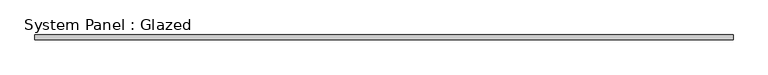
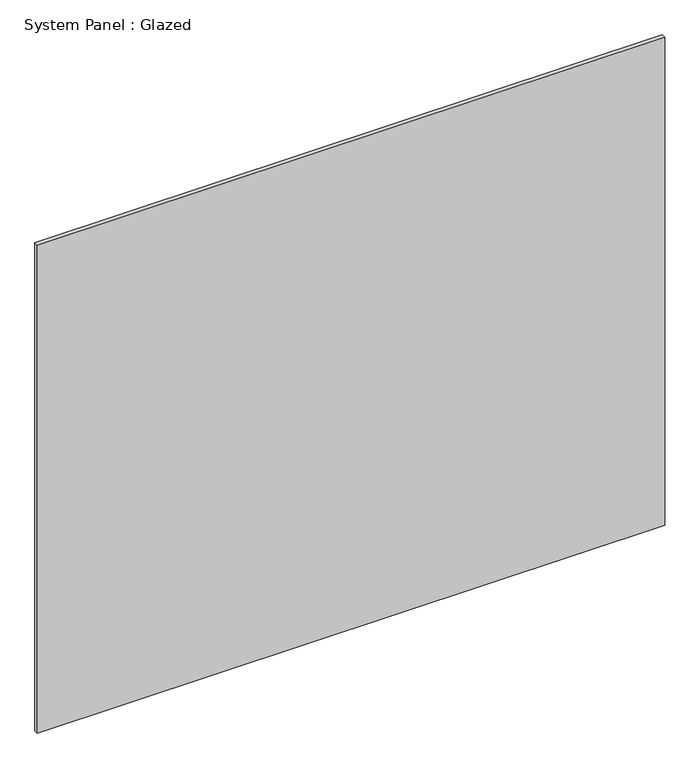
"""IFC4 building model written with IfcOpenShell, lengths in millimetres: plate geometry, System Panel : Glazed."""

from ifc_helpers import new_model, si_unit, origin, origin_with_axes, place, context, project, spatial, polyline, outline, extrude, source, transform, mapped, element, save


def system_panel_glazed_4ffbc40e(model_context):
    return source(origin(), model_context, "Body", "SweptSolid", [
        extrude(outline(polyline([(1776.2508233, 19.05), (-1776.2508233, 19.05), (-1776.2508233, 44.45), (1776.2508233, 44.45), (1776.2508233, 19.05)])), origin_with_axes(), (0.0, 0.0, 1.0), 2921.0),
    ])


if __name__ == "__main__":
    model = new_model("IFC4")
    model_context = context("Model", 3, world=origin())
    ifc_project = project(units=[si_unit("LENGTHUNIT", "METRE", prefix="MILLI")], contexts=[model_context])
    site = spatial("IfcSite", under=ifc_project)
    building = spatial("IfcBuilding", under=site)
    placement = place(None, origin())
    system_panel_glazed_shape = system_panel_glazed_4ffbc40e(model_context)
    element("IfcPlate", 1, ObjectType="System Panel : Glazed", at=placement, inside=building, context=model_context, shape_type="MappedRepresentation", body=[
        mapped(system_panel_glazed_shape, transform((0.0, 0.0, 0.0), x_axis=(1.0, 0.0, 0.0), y_axis=(0.0, 1.0, 0.0), z_axis=(0.0, 0.0, 1.0))),
    ])
    save(model, "model.ifc")

# Revit data of these elements
# Type "System Panel : Glazed"
#   Construction Type Id = "GSP4R"
#   Analytic Construction = "1/8 in Pilkington single glazing"
#   Visual Light Transmittance = 0.9
#   Solar Heat Gain Coefficient = 0.86
#   Heat Transfer Coefficient (U) = 1.18115 BTU/(h·ft²·°F)
#   Define Thermal Properties by = 1
# Element 1 (IfcPlate, "System Panel : Glazed")
#   Materials on its faces: "Glass"
# Materials
#   "Glass": class "Glass", colour RGB 0 128 192, transparency 0.75, Description = "Soda Lime Glass", Cost = 0
